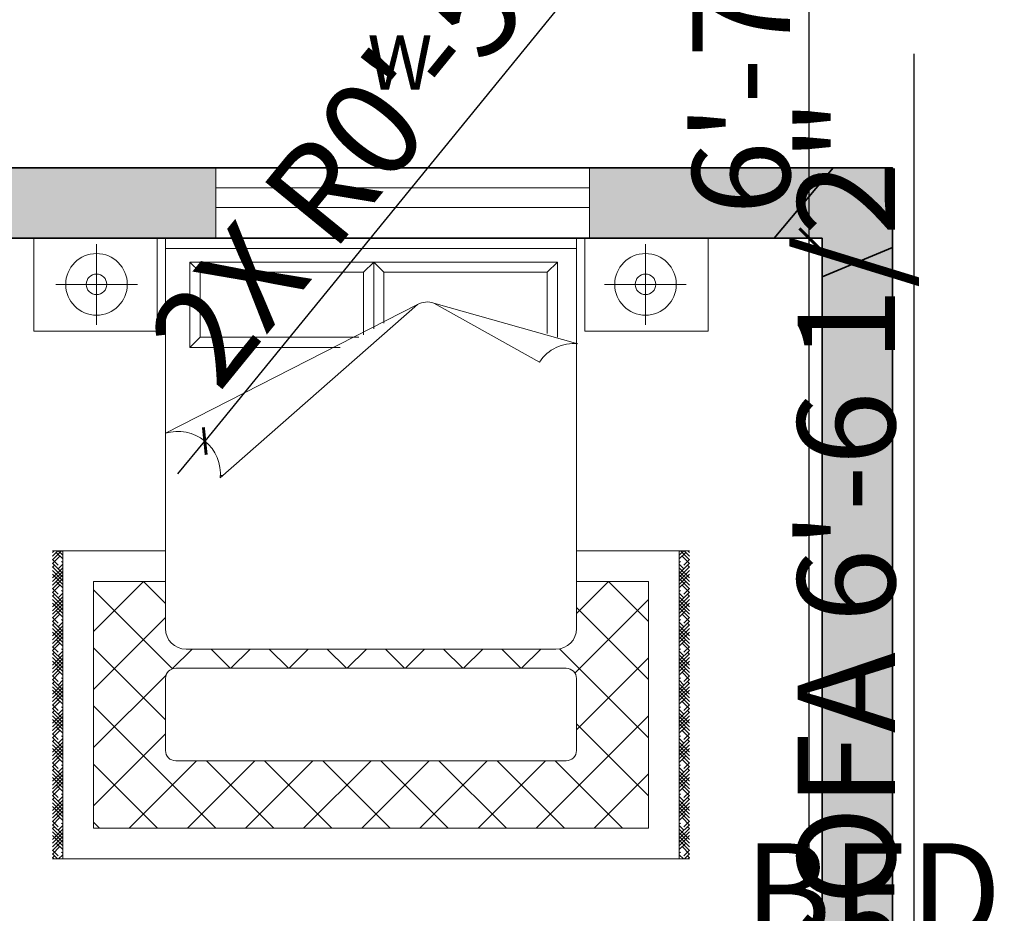
# Model space of a CAD drawing. Units: inches. Extents: x 1858 to 2399, y 1317 to 1943.
# Tile 6 of 8: x 2162 to 2288, y 1742 to 1856. Entities that reach past the tile are written whole.
import ezdxf

# ---------------------------------------------------------------- set-up
doc = ezdxf.new("R2010")
doc.units = ezdxf.units.IN
for name, color, linetype, lineweight in [('A-ANNO-DIMS', 2, 'Continuous', 18), ('A-ANNO-TEXT', 7, 'Continuous', 18), ('A-COLS', 7, 'Continuous', 35), ('A-COLS-PATT', 5, 'Continuous', 13), ('A-WALL', 7, 'Continuous', 35), ('A-WALL-PATT', 1, 'Continuous', 13), ('beds', 15, 'Continuous', 18), ('window', 4, 'Continuous', 18)]:
    doc.layers.add(name, color=color, linetype=linetype, lineweight=lineweight)
doc.styles.get("Standard").update_dxf_attribs({"font": 'arial.ttf'})
doc.dimstyles.new('ISO-25', dxfattribs={"dimtxt": 12.5, "dimasz": 2.5, "dimexe": 1.25, "dimexo": 0.625, "dimtad": 1, "dimdec": 0, "dimlunit": 4, "dimtxsty": 'Standard', "dimblk": 'ARCHTICK', "dimcen": 2.5, "dimse1": 1, "dimse2": 1, "dimclrd": 3, "dimclrt": 4, "dimadec": 0, "dimazin": 0, "dimtfac": 1, "dimtdec": 0, "dimtmove": 0, "dimatfit": 3, "dimfxl": 1, "dimarcsym": 0})

# ---------------------------------------------------------------- blocks, each defined once
blk = doc.blocks.new('A$C4CB008C5')
for p, q in [((0, 3.0188), (0.6, 3.0188)), ((0, 2.5688), (0, 3.0188)), ((0.6, 3.0188), (0.6, 2.5688)), ((0.6397, 1.1213), (0.6397, 3.0213)), ((0.6397, 3.0213), (2.6397, 3.0213)), ((2.6397, 3.0213), (2.6397, 1.1213)), ((3.2794, 3.0188), (2.6794, 3.0188)), ((2.6794, 3.0188), (2.6794, 2.5688)), ((3.2794, 2.5688), (3.2794, 3.0188)), ((0.3042, 2.5999), (0.3042, 2.9921)), ((0.6397, 2.9713), (2.6397, 2.9713)), ((2.9753, 2.5999), (2.9753, 2.9921)), ((0.7588, 2.9048), (2.5468, 2.9048)), ((0.7588, 2.4886), (0.7588, 2.9048)), ((0.7588, 2.9048), (0.8088, 2.8548)), ((1.6028, 2.8548), (1.6528, 2.9048)), ((1.6528, 2.9048), (1.6528, 2.5791)), ((1.6528, 2.9048), (1.7028, 2.8548)), ((2.4968, 2.8548), (2.5468, 2.9048)), ((2.5468, 2.9048), (2.5468, 2.5398)), ((0.8088, 2.8548), (1.6028, 2.8548)), ((0.8088, 2.5386), (0.8088, 2.8548)), ((1.6028, 2.8548), (1.6028, 2.5513)), ((1.7028, 2.8548), (1.7028, 2.6069)), ((1.7028, 2.8548), (2.4968, 2.8548)), ((2.4968, 2.8548), (2.4968, 2.5563)), ((0.1057, 2.796), (0.5033, 2.796)), ((3.1738, 2.796), (2.7761, 2.796)), ((0.6397, 2.0713), (1.866, 2.6977)), ((0.9063, 1.8539), (1.866, 2.6977)), ((1.946, 2.7052), (2.6461, 2.507)), ((1.946, 2.7052), (2.4598, 2.4178)), ((0.6, 2.5688), (0, 2.5688)), ((2.6794, 2.5688), (3.2794, 2.5688)), ((0.8088, 2.5386), (0.7588, 2.4886)), ((1.58, 2.5386), (0.8088, 2.5386)), ((1.4901, 2.4886), (0.7588, 2.4886)), ((0.9071, 1.8666), (0.9192, 1.8666)), ((0.0897, 1.5), (0.6397, 1.5)), ((0.0897, 1.491), (0.0987, 1.5)), ((0.0897, 1.4733), (0.1164, 1.5)), ((0.0897, 1.4557), (0.1341, 1.5)), ((0.1397, 1.4602), (0.1081, 1.4917)), ((0.1397, 1.4778), (0.1175, 1.5)), ((0.1397, 1.4955), (0.1352, 1.5)), ((0.1397, 0), (0.1397, 1.5)), ((2.6397, 1.5), (3.1897, 1.5)), ((3.1397, 1.4955), (3.1442, 1.5)), ((3.1397, 1.4778), (3.1619, 1.5)), ((3.1397, 1.5), (3.1397, 0)), ((3.1397, 1.4602), (3.1713, 1.4917)), ((3.1897, 1.4557), (3.1454, 1.5)), ((3.1897, 1.4733), (3.163, 1.5)), ((3.1897, 1.491), (3.1807, 1.5)), ((0.0904, 1.4741), (0.0897, 1.4748)), ((0.0897, 1.438), (0.1258, 1.4741)), ((0.117, 1.4299), (0.0897, 1.4571)), ((0.1397, 1.3894), (0.0897, 1.4394)), ((0.1397, 1.4425), (0.1346, 1.4475)), ((3.1397, 1.4425), (3.1448, 1.4475)), ((3.1397, 1.3894), (3.1897, 1.4394)), ((3.1897, 1.438), (3.1536, 1.4741)), ((3.1625, 1.4299), (3.1897, 1.4571)), ((3.189, 1.4741), (3.1897, 1.4748)), ((0.0897, 1.4203), (0.0993, 1.4299)), ((0.1397, 1.3718), (0.0897, 1.4218)), ((0.1397, 1.3541), (0.0897, 1.4041)), ((0.0897, 1.3496), (0.1397, 1.3996)), ((0.0904, 1.368), (0.1397, 1.4173)), ((0.117, 1.4122), (0.1397, 1.4349)), ((3.1625, 1.4122), (3.1397, 1.4349)), ((3.1397, 1.3718), (3.1897, 1.4218)), ((3.189, 1.368), (3.1397, 1.4173)), ((3.1397, 1.3541), (3.1897, 1.4041)), ((3.1897, 1.3496), (3.1397, 1.3996)), ((3.1897, 1.4203), (3.1801, 1.4299)), ((0.1397, 1.3364), (0.0897, 1.3864)), ((0.0897, 1.3319), (0.1397, 1.3819)), ((0.0897, 1.3142), (0.1397, 1.3642)), ((0.1397, 1.3187), (0.1081, 1.3503)), ((0.2897, 1.1076), (0.5321, 1.35)), ((0.2897, 0.15), (0.2897, 1.35)), ((0.2897, 1.35), (0.6397, 1.35)), ((0.6397, 1.243), (0.5327, 1.35)), ((2.6397, 1.1949), (2.7948, 1.35)), ((2.6397, 1.35), (2.9897, 1.35)), ((2.9897, 1.1557), (2.7955, 1.35)), ((2.9897, 1.35), (2.9897, 0.15)), ((3.1397, 1.3364), (3.1897, 1.3864)), ((3.1897, 1.3319), (3.1397, 1.3819)), ((3.1897, 1.3142), (3.1397, 1.3642)), ((3.1397, 1.3187), (3.1713, 1.3503)), ((0.0904, 1.3326), (0.0897, 1.3334)), ((0.0897, 1.2966), (0.1258, 1.3326)), ((0.117, 1.2885), (0.0897, 1.3157)), ((0.1397, 1.248), (0.0897, 1.298)), ((0.117, 1.2708), (0.1397, 1.2935)), ((0.1397, 1.3011), (0.1346, 1.3061)), ((0.6743, 0.9255), (0.2897, 1.3102)), ((3.1397, 1.3011), (3.1448, 1.3061)), ((3.1397, 1.248), (3.1897, 1.298)), ((3.1625, 1.2708), (3.1397, 1.2935)), ((3.1897, 1.2966), (3.1536, 1.3326)), ((3.1625, 1.2885), (3.1897, 1.3157)), ((3.189, 1.3326), (3.1897, 1.3334)), ((0.0897, 1.2789), (0.0993, 1.2885)), ((0.1397, 1.2303), (0.0897, 1.2803)), ((0.1397, 1.2127), (0.0897, 1.2627)), ((0.0897, 1.2082), (0.1397, 1.2582)), ((0.0904, 1.2266), (0.1397, 1.2758)), ((2.6321, 0.9045), (2.9897, 1.2621)), ((3.1397, 1.2303), (3.1897, 1.2803)), ((3.189, 1.2266), (3.1397, 1.2758)), ((3.1397, 1.2127), (3.1897, 1.2627)), ((3.1897, 1.2082), (3.1397, 1.2582)), ((3.1897, 1.2789), (3.1801, 1.2885)), ((0.1397, 1.195), (0.0897, 1.245)), ((0.0897, 1.1905), (0.1397, 1.2405)), ((0.0897, 1.1728), (0.1397, 1.2228)), ((0.1397, 1.1773), (0.1081, 1.2089)), ((2.9897, 0.8729), (2.6397, 1.2229)), ((3.1397, 1.195), (3.1897, 1.245)), ((3.1897, 1.1905), (3.1397, 1.2405)), ((3.1897, 1.1728), (3.1397, 1.2228)), ((3.1397, 1.1773), (3.1713, 1.2089)), ((0.0904, 1.1912), (0.0897, 1.192)), ((0.0897, 1.1551), (0.1258, 1.1912)), ((0.117, 1.147), (0.0897, 1.1743)), ((0.1397, 1.1066), (0.0897, 1.1566)), ((0.117, 1.1294), (0.1397, 1.1521)), ((0.1397, 1.1596), (0.1346, 1.1647)), ((0.2897, 0.8248), (0.6397, 1.1748)), ((3.1397, 1.1596), (3.1448, 1.1647)), ((3.1397, 1.1066), (3.1897, 1.1566)), ((3.1625, 1.1294), (3.1397, 1.1521)), ((3.1897, 1.1551), (3.1536, 1.1912)), ((3.1625, 1.147), (3.1897, 1.1743)), ((3.189, 1.1912), (3.1897, 1.192)), ((0.0897, 1.1375), (0.0993, 1.147)), ((0.1397, 1.0889), (0.0897, 1.1389)), ((0.1397, 1.0712), (0.0897, 1.1212)), ((0.0897, 1.0667), (0.1397, 1.1167)), ((0.1397, 1.0536), (0.0897, 1.1036)), ((0.0904, 1.0852), (0.1397, 1.1344)), ((3.1397, 1.0889), (3.1897, 1.1389)), ((3.189, 1.0852), (3.1397, 1.1344)), ((3.1397, 1.0712), (3.1897, 1.1212)), ((3.1897, 1.0667), (3.1397, 1.1167)), ((3.1397, 1.0536), (3.1897, 1.1036)), ((3.1897, 1.1375), (3.1801, 1.147)), ((0.0897, 1.0491), (0.1397, 1.0991)), ((0.0897, 1.0314), (0.1397, 1.0814)), ((0.1397, 1.0359), (0.1081, 1.0675)), ((3.1897, 1.0491), (3.1397, 1.0991)), ((3.1897, 1.0314), (3.1397, 1.0814)), ((3.1397, 1.0359), (3.1713, 1.0675)), ((0.0904, 1.0498), (0.0897, 1.0505)), ((0.0897, 1.0137), (0.1258, 1.0498)), ((0.117, 1.0056), (0.0897, 1.0329)), ((0.1397, 0.9652), (0.0897, 1.0152)), ((0.117, 0.9879), (0.1397, 1.0107)), ((0.1397, 1.0182), (0.1346, 1.0233)), ((0.6397, 0.6773), (0.2897, 1.0273)), ((0.6727, 0.925), (0.769, 1.0213)), ((2.5397, 1.0213), (0.7397, 1.0213)), ((0.9548, 0.9279), (0.8614, 1.0213)), ((0.9585, 0.9279), (1.0519, 1.0213)), ((1.2376, 0.9279), (1.1443, 1.0213)), ((1.2414, 0.9279), (1.3347, 1.0213)), ((1.5205, 0.9279), (1.4271, 1.0213)), ((1.5242, 0.9279), (1.6176, 1.0213)), ((1.8033, 0.9279), (1.71, 1.0213)), ((1.8071, 0.9279), (1.9004, 1.0213)), ((2.0861, 0.9279), (1.9928, 1.0213)), ((2.0899, 0.9279), (2.1832, 1.0213)), ((2.369, 0.9279), (2.2757, 1.0213)), ((2.3727, 0.9279), (2.4661, 1.0213)), ((2.9897, 0.5901), (2.557, 1.0228)), ((3.1397, 1.0182), (3.1448, 1.0233)), ((3.1397, 0.9652), (3.1897, 1.0152)), ((3.1625, 0.9879), (3.1397, 1.0107)), ((3.1897, 1.0137), (3.1536, 1.0498)), ((3.1625, 1.0056), (3.1897, 1.0329)), ((3.189, 1.0498), (3.1897, 1.0505)), ((0.0897, 0.996), (0.0993, 1.0056)), ((0.1397, 0.9475), (0.0897, 0.9975)), ((0.1397, 0.9298), (0.0897, 0.9798)), ((0.0897, 0.9253), (0.1397, 0.9753)), ((0.1397, 0.9121), (0.0897, 0.9621)), ((0.0904, 0.9437), (0.1397, 0.993)), ((2.6397, 0.6292), (2.9897, 0.9792)), ((3.1397, 0.9475), (3.1897, 0.9975)), ((3.189, 0.9437), (3.1397, 0.993)), ((3.1397, 0.9298), (3.1897, 0.9798)), ((3.1897, 0.9253), (3.1397, 0.9753)), ((3.1397, 0.9121), (3.1897, 0.9621)), ((3.1897, 0.996), (3.1801, 1.0056)), ((0.0897, 0.9076), (0.1397, 0.9576)), ((0.0897, 0.89), (0.1397, 0.94)), ((0.1397, 0.8945), (0.1081, 0.9261)), ((0.6897, 0.9279), (2.5897, 0.9279)), ((3.1897, 0.9076), (3.1397, 0.9576)), ((3.1897, 0.89), (3.1397, 0.94)), ((3.1397, 0.8945), (3.1713, 0.9261)), ((0.0904, 0.9084), (0.0897, 0.9091)), ((0.0897, 0.8723), (0.1258, 0.9084)), ((0.117, 0.8642), (0.0897, 0.8914)), ((0.1397, 0.8238), (0.0897, 0.8738)), ((0.0897, 0.8546), (0.0993, 0.8642)), ((0.117, 0.8465), (0.1397, 0.8693)), ((0.1397, 0.8768), (0.1346, 0.8819)), ((0.2897, 0.542), (0.6427, 0.8949)), ((0.6397, 0.8779), (0.6397, 0.5279)), ((2.6397, 0.8779), (2.6397, 0.5279)), ((3.1397, 0.8768), (3.1448, 0.8819)), ((3.1397, 0.8238), (3.1897, 0.8738)), ((3.1625, 0.8465), (3.1397, 0.8693)), ((3.1897, 0.8723), (3.1536, 0.9084)), ((3.1625, 0.8642), (3.1897, 0.8914)), ((3.1897, 0.8546), (3.1801, 0.8642)), ((3.189, 0.9084), (3.1897, 0.9091)), ((0.1397, 0.8061), (0.0897, 0.8561)), ((0.1397, 0.7884), (0.0897, 0.8384)), ((0.0897, 0.7839), (0.1397, 0.8339)), ((0.1397, 0.7707), (0.0897, 0.8207)), ((0.0897, 0.7662), (0.1397, 0.8162)), ((0.0904, 0.8023), (0.1397, 0.8516)), ((3.1397, 0.8061), (3.1897, 0.8561)), ((3.189, 0.8023), (3.1397, 0.8516)), ((3.1397, 0.7884), (3.1897, 0.8384)), ((3.1897, 0.7839), (3.1397, 0.8339)), ((3.1397, 0.7707), (3.1897, 0.8207)), ((3.1897, 0.7662), (3.1397, 0.8162)), ((0.0897, 0.7485), (0.1397, 0.7985)), ((0.0904, 0.767), (0.0897, 0.7677)), ((0.0897, 0.7309), (0.1258, 0.767)), ((0.1397, 0.7531), (0.1081, 0.7846)), ((3.1897, 0.7485), (3.1397, 0.7985)), ((3.1397, 0.7531), (3.1713, 0.7846)), ((3.1897, 0.7309), (3.1536, 0.767)), ((3.189, 0.767), (3.1897, 0.7677)), ((0.117, 0.7228), (0.0897, 0.75)), ((0.1397, 0.6823), (0.0897, 0.7323)), ((0.0897, 0.7132), (0.0993, 0.7228)), ((0.117, 0.7051), (0.1397, 0.7278)), ((0.1397, 0.7354), (0.1346, 0.7404)), ((0.8842, 0.15), (0.2897, 0.7445)), ((3.1397, 0.7354), (3.1448, 0.7404)), ((3.1397, 0.6823), (3.1897, 0.7323)), ((3.1625, 0.7051), (3.1397, 0.7278)), ((3.1625, 0.7228), (3.1897, 0.75)), ((3.1897, 0.7132), (3.1801, 0.7228)), ((0.1397, 0.6647), (0.0897, 0.7147)), ((0.1397, 0.647), (0.0897, 0.697)), ((0.0897, 0.6425), (0.1397, 0.6925)), ((0.1397, 0.6293), (0.0897, 0.6793)), ((0.0897, 0.6248), (0.1397, 0.6748)), ((0.0904, 0.6609), (0.1397, 0.7102)), ((2.4433, 0.15), (2.9897, 0.6964)), ((3.1397, 0.6647), (3.1897, 0.7147)), ((3.189, 0.6609), (3.1397, 0.7102)), ((3.1397, 0.647), (3.1897, 0.697)), ((3.1897, 0.6425), (3.1397, 0.6925)), ((3.1397, 0.6293), (3.1897, 0.6793)), ((3.1897, 0.6248), (3.1397, 0.6748)), ((0.0897, 0.6071), (0.1397, 0.6571)), ((0.0904, 0.6255), (0.0897, 0.6263)), ((0.0897, 0.5894), (0.1258, 0.6255)), ((0.1397, 0.6116), (0.1081, 0.6432)), ((2.9897, 0.3072), (2.6397, 0.6572)), ((3.1897, 0.6071), (3.1397, 0.6571)), ((3.1397, 0.6116), (3.1713, 0.6432)), ((3.1897, 0.5894), (3.1536, 0.6255)), ((3.189, 0.6255), (3.1897, 0.6263)), ((0.117, 0.5813), (0.0897, 0.6086)), ((0.1397, 0.5409), (0.0897, 0.5909)), ((0.0897, 0.5718), (0.0993, 0.5813)), ((0.117, 0.5637), (0.1397, 0.5864)), ((0.1397, 0.594), (0.1346, 0.599)), ((0.2897, 0.2591), (0.6397, 0.6091)), ((3.1397, 0.594), (3.1448, 0.599)), ((3.1397, 0.5409), (3.1897, 0.5909)), ((3.1625, 0.5637), (3.1397, 0.5864)), ((3.1625, 0.5813), (3.1897, 0.6086)), ((3.1897, 0.5718), (3.1801, 0.5813)), ((0.1397, 0.5232), (0.0897, 0.5732)), ((0.1397, 0.5056), (0.0897, 0.5556)), ((0.0897, 0.5011), (0.1397, 0.5511)), ((0.1397, 0.4879), (0.0897, 0.5379)), ((0.0897, 0.4834), (0.1397, 0.5334)), ((0.0904, 0.5195), (0.1397, 0.5687)), ((3.1397, 0.5232), (3.1897, 0.5732)), ((3.189, 0.5195), (3.1397, 0.5687)), ((3.1397, 0.5056), (3.1897, 0.5556)), ((3.1897, 0.5011), (3.1397, 0.5511)), ((3.1397, 0.4879), (3.1897, 0.5379)), ((3.1897, 0.4834), (3.1397, 0.5334)), ((0.0897, 0.4657), (0.1397, 0.5157)), ((0.0904, 0.4841), (0.0897, 0.4849)), ((0.0897, 0.448), (0.1258, 0.4841)), ((0.1397, 0.4702), (0.1081, 0.5018)), ((3.1897, 0.4657), (3.1397, 0.5157)), ((3.1397, 0.4702), (3.1713, 0.5018)), ((3.1897, 0.448), (3.1536, 0.4841)), ((3.189, 0.4841), (3.1897, 0.4849)), ((0.117, 0.4399), (0.0897, 0.4672)), ((0.1397, 0.3995), (0.0897, 0.4495)), ((0.0897, 0.4303), (0.0993, 0.4399)), ((0.1397, 0.3818), (0.0897, 0.4318)), ((0.117, 0.4222), (0.1397, 0.445)), ((0.1397, 0.4525), (0.1346, 0.4576)), ((0.6013, 0.15), (0.2897, 0.4616)), ((0.4634, 0.15), (0.7914, 0.4779)), ((0.6897, 0.4779), (2.5897, 0.4779)), ((0.7463, 0.15), (1.0742, 0.4779)), ((1.167, 0.15), (0.8391, 0.4779)), ((1.0291, 0.15), (1.3571, 0.4779)), ((1.4499, 0.15), (1.1219, 0.4779)), ((1.312, 0.15), (1.6399, 0.4779)), ((1.7327, 0.15), (1.4048, 0.4779)), ((1.5948, 0.15), (1.9227, 0.4779)), ((2.0156, 0.15), (1.6876, 0.4779)), ((1.8777, 0.15), (2.2056, 0.4779)), ((2.2984, 0.15), (1.9705, 0.4779)), ((2.1605, 0.15), (2.4884, 0.4779)), ((2.5812, 0.15), (2.2533, 0.4779)), ((2.8641, 0.15), (2.5361, 0.4779)), ((3.1397, 0.4525), (3.1448, 0.4576)), ((3.1397, 0.3995), (3.1897, 0.4495)), ((3.1625, 0.4222), (3.1397, 0.445)), ((3.1397, 0.3818), (3.1897, 0.4318)), ((3.1625, 0.4399), (3.1897, 0.4672)), ((3.1897, 0.4303), (3.1801, 0.4399)), ((0.1397, 0.3641), (0.0897, 0.4141)), ((0.0897, 0.3596), (0.1397, 0.4096)), ((0.1397, 0.3465), (0.0897, 0.3965)), ((0.0897, 0.342), (0.1397, 0.392)), ((0.0904, 0.3781), (0.1397, 0.4273)), ((2.7262, 0.15), (2.9897, 0.4135)), ((3.189, 0.3781), (3.1397, 0.4273)), ((3.1397, 0.3641), (3.1897, 0.4141)), ((3.1897, 0.3596), (3.1397, 0.4096)), ((3.1397, 0.3465), (3.1897, 0.3965)), ((3.1897, 0.342), (3.1397, 0.392)), ((0.0897, 0.3243), (0.1397, 0.3743)), ((0.0904, 0.3427), (0.0897, 0.3434)), ((0.0897, 0.3066), (0.1258, 0.3427)), ((0.1397, 0.3288), (0.1081, 0.3604)), ((3.1897, 0.3243), (3.1397, 0.3743)), ((3.1397, 0.3288), (3.1713, 0.3604)), ((3.1897, 0.3066), (3.1536, 0.3427)), ((3.189, 0.3427), (3.1897, 0.3434)), ((0.117, 0.2985), (0.0897, 0.3258)), ((0.1397, 0.2581), (0.0897, 0.3081)), ((0.0897, 0.2889), (0.0993, 0.2985)), ((0.1397, 0.2404), (0.0897, 0.2904)), ((0.117, 0.2808), (0.1397, 0.3036)), ((0.1397, 0.3111), (0.1346, 0.3162)), ((3.1397, 0.3111), (3.1448, 0.3162)), ((3.1397, 0.2581), (3.1897, 0.3081)), ((3.1625, 0.2808), (3.1397, 0.3036)), ((3.1397, 0.2404), (3.1897, 0.2904)), ((3.1625, 0.2985), (3.1897, 0.3258)), ((3.1897, 0.2889), (3.1801, 0.2985)), ((0.1397, 0.2227), (0.0897, 0.2727)), ((0.0897, 0.2182), (0.1397, 0.2682)), ((0.1397, 0.205), (0.0897, 0.255)), ((0.0897, 0.2005), (0.1397, 0.2505)), ((0.0904, 0.2366), (0.1397, 0.2859)), ((3.189, 0.2366), (3.1397, 0.2859)), ((3.1397, 0.2227), (3.1897, 0.2727)), ((3.1897, 0.2182), (3.1397, 0.2682)), ((3.1397, 0.205), (3.1897, 0.255)), ((3.1897, 0.2005), (3.1397, 0.2505)), ((0.0897, 0.1829), (0.1397, 0.2329)), ((0.0904, 0.2013), (0.0897, 0.202)), ((0.0897, 0.1652), (0.1258, 0.2013)), ((0.1397, 0.1874), (0.1081, 0.219)), ((3.1897, 0.1829), (3.1397, 0.2329)), ((3.1397, 0.1874), (3.1713, 0.219)), ((3.1897, 0.1652), (3.1536, 0.2013)), ((3.189, 0.2013), (3.1897, 0.202)), ((0.117, 0.1571), (0.0897, 0.1843)), ((0.1397, 0.1167), (0.0897, 0.1667)), ((0.0897, 0.1475), (0.0993, 0.1571)), ((0.1397, 0.099), (0.0897, 0.149)), ((0.0904, 0.0952), (0.1397, 0.1445)), ((0.117, 0.1394), (0.1397, 0.1621)), ((0.1397, 0.1697), (0.1346, 0.1748)), ((0.3185, 0.15), (0.2897, 0.1788)), ((2.9897, 0.15), (0.2897, 0.15)), ((3.1397, 0.1697), (3.1448, 0.1748)), ((3.1397, 0.1167), (3.1897, 0.1667)), ((3.1625, 0.1394), (3.1397, 0.1621)), ((3.1397, 0.099), (3.1897, 0.149)), ((3.189, 0.0952), (3.1397, 0.1445)), ((3.1625, 0.1571), (3.1897, 0.1843)), ((3.1897, 0.1475), (3.1801, 0.1571)), ((0.1397, 0.0813), (0.0897, 0.1313)), ((0.0897, 0.0768), (0.1397, 0.1268)), ((0.1397, 0.0636), (0.0897, 0.1136)), ((0.0897, 0.0591), (0.1397, 0.1091)), ((3.1397, 0.0813), (3.1897, 0.1313)), ((3.1897, 0.0768), (3.1397, 0.1268)), ((3.1397, 0.0636), (3.1897, 0.1136)), ((3.1897, 0.0591), (3.1397, 0.1091)), ((0.0897, 0.0414), (0.1397, 0.0914)), ((0.0904, 0.0599), (0.0897, 0.0606)), ((0.0897, 0.0238), (0.1258, 0.0599)), ((0.1397, 0.0459), (0.1081, 0.0775)), ((3.1897, 0.0414), (3.1397, 0.0914)), ((3.1397, 0.0459), (3.1713, 0.0775)), ((3.1897, 0.0238), (3.1536, 0.0599)), ((3.189, 0.0599), (3.1897, 0.0606)), ((0.117, 0.0157), (0.0897, 0.0429)), ((0.1149, 0), (0.0897, 0.0252)), ((0.0897, 0.0061), (0.0993, 0.0157)), ((0.0973, 0), (0.0897, 0.0076)), ((0.119, 0), (0.1397, 0.0207)), ((0.1397, 0.0283), (0.1346, 0.0333)), ((0.1367, 0), (0.1397, 0.0031)), ((3.1397, 0.0283), (3.1448, 0.0333)), ((3.1604, 0), (3.1397, 0.0207)), ((3.1428, 0), (3.1397, 0.0031)), ((3.1625, 0.0157), (3.1897, 0.0429)), ((3.1645, 0), (3.1897, 0.0252)), ((3.1897, 0.0061), (3.1801, 0.0157)), ((3.1822, 0), (3.1897, 0.0076)), ((0.0897, 0), (3.1897, 0))]:
    blk.add_line(p, q)
for centre, radius in [((0.3042, 2.796), 0.15), ((2.9753, 2.796), 0.15), ((0.3042, 2.796), 0.05), ((2.9753, 2.796), 0.05)]:
    blk.add_circle(centre, radius)
for centre, radius, start, end in [((1.9146, 2.6103), 0.1, 71.7215, 119.0799), ((2.626, 2.3098), 0.1982, 84.1725, 146.9889), ((0.7002, 1.8733), 0.207, 354.6422, 106.9775), ((0.7397, 1.1213), 0.1, 180, 270), ((2.5397, 1.1213), 0.1, 270, 0), ((0.6897, 0.8779), 0.05, 90, 180), ((2.5897, 0.8779), 0.05, 0, 90), ((0.6897, 0.5279), 0.05, 180, 270), ((2.5897, 0.5279), 0.05, 270, 0)]:
    blk.add_arc(centre, radius, start, end)
blk = doc.blocks.new('_ArchTick')
at = {"color": 0, "linetype": 'ByBlock', "const_width": 0.15}
blk.add_lwpolyline([(-0.5, -0.5), (0.5, 0.5)], dxfattribs=at)
blk = doc.blocks.new('*D13')
at = {"layer": 'A-ANNO-DIMS', "color": 0, "lineweight": -2, "transparency": 16777216}
blk.add_line((2316.13, 1837.34), (2316.13, 1357.34), dxfattribs=at)
at = {"layer": 'Defpoints', "color": 0, "transparency": 16777216}
for p in [(2273.38, 1837.34), (2273.38, 1357.34), (2316.13, 1357.34)]:
    blk.add_point(p, dxfattribs=at)
at = {"layer": 'A-ANNO-DIMS', "color": 0, "lineweight": -2, "transparency": 16777216, "xscale": 2.5, "yscale": 2.5, "zscale": 2.5}
for p, rotation in [((2316.13, 1837.34), 90), ((2316.13, 1357.34), 270)]:
    blk.add_blockref('_ArchTick', p, dxfattribs=dict(at, rotation=rotation))
at = {"layer": 'A-ANNO-DIMS', "color": 0, "transparency": 16777216, "insert": (2309.12, 1597.34), "char_height": 12.5, "attachment_point": 5, "rotation": 90}
blk.add_mtext("40'", dxfattribs=at)
blk = doc.blocks.new('*D14')
at = {"layer": 'A-ANNO-DIMS', "color": 0, "lineweight": -2, "transparency": 16777216}
blk.add_line((1913.38, 1886.42), (2273.38, 1886.42), dxfattribs=at)
at = {"layer": 'Defpoints', "color": 0, "transparency": 16777216}
for p in [(2273.38, 1886.42), (1913.38, 1826.41), (2273.38, 1827.14)]:
    blk.add_point(p, dxfattribs=at)
at = {"layer": 'A-ANNO-DIMS', "color": 0, "lineweight": -2, "transparency": 16777216, "xscale": 2.5, "yscale": 2.5, "zscale": 2.5, "rotation": 180}
blk.add_blockref('_ArchTick', (1913.38, 1886.42), dxfattribs=at)
at = {"layer": 'A-ANNO-DIMS', "color": 0, "lineweight": -2, "transparency": 16777216, "xscale": 2.5, "yscale": 2.5, "zscale": 2.5}
blk.add_blockref('_ArchTick', (2273.38, 1886.42), dxfattribs=at)
at = {"layer": 'A-ANNO-DIMS', "color": 0, "transparency": 16777216, "insert": (2093.38, 1893.43), "char_height": 12.5, "attachment_point": 5}
blk.add_mtext("30'", dxfattribs=at)
blk = doc.blocks.new('*D15')
at = {"layer": 'A-ANNO-DIMS', "color": 3, "lineweight": -2, "transparency": 16777216}
for p, q in [((2163.42, 1735.85), (2249.76, 1735.85)), ((2249.76, 1735.85), (2399.03, 1735.85))]:
    blk.add_line(p, q, dxfattribs=at)
at = {"layer": 'Defpoints', "color": 0, "transparency": 16777216}
for p in [(2163.42, 1748.8), (2249.76, 1748.8), (2249.76, 1735.85)]:
    blk.add_point(p, dxfattribs=at)
at = {"layer": 'A-ANNO-DIMS', "color": 3, "lineweight": -2, "transparency": 16777216, "xscale": 2.5, "yscale": 2.5, "zscale": 2.5, "rotation": 180}
blk.add_blockref('_ArchTick', (2163.42, 1735.85), dxfattribs=at)
at = {"layer": 'A-ANNO-DIMS', "color": 3, "lineweight": -2, "transparency": 16777216, "xscale": 2.5, "yscale": 2.5, "zscale": 2.5}
blk.add_blockref('_ArchTick', (2249.76, 1735.85), dxfattribs=at)
at = {"layer": 'A-ANNO-DIMS', "color": 4, "transparency": 16777216, "insert": (2325.64, 1742.94), "char_height": 12.5, "attachment_point": 5}
blk.add_mtext('BED 7\'-2 1/2" TYP.', dxfattribs=at)
blk = doc.blocks.new('*D16')
at = {"layer": 'A-ANNO-DIMS', "color": 3, "lineweight": -2, "transparency": 16777216}
for p, q in [((2262.71, 1828.34), (2262.71, 1937.48)), ((2262.71, 1748.8), (2262.71, 1828.34))]:
    blk.add_line(p, q, dxfattribs=at)
at = {"layer": 'Defpoints', "color": 0, "transparency": 16777216}
for p in [(2249.76, 1828.34), (2262.71, 1828.34), (2249.76, 1748.8)]:
    blk.add_point(p, dxfattribs=at)
at = {"layer": 'A-ANNO-DIMS', "color": 3, "lineweight": -2, "transparency": 16777216, "xscale": 2.5, "yscale": 2.5, "zscale": 2.5}
for p, rotation in [((2262.71, 1828.34), 90), ((2262.71, 1748.8), 270)]:
    blk.add_blockref('_ArchTick', p, dxfattribs=dict(at, rotation=rotation))
at = {"layer": 'A-ANNO-DIMS', "color": 4, "transparency": 16777216, "insert": (2255.62, 1884.16), "char_height": 12.5, "attachment_point": 5, "rotation": 90}
blk.add_mtext('6\'-7 1/2" TYP.', dxfattribs=at)
blk = doc.blocks.new('*D17')
at = {"layer": 'A-ANNO-DIMS', "color": 3, "lineweight": -2, "transparency": 16777216}
for p, q in [((2276.18, 1653.07), (2276.18, 1851.95)), ((2276.18, 1574.39), (2276.18, 1653.07))]:
    blk.add_line(p, q, dxfattribs=at)
at = {"layer": 'Defpoints', "color": 0, "transparency": 16777216}
for p in [(2264.38, 1653.07), (2276.18, 1653.07), (2264.38, 1574.39)]:
    blk.add_point(p, dxfattribs=at)
at = {"layer": 'A-ANNO-DIMS', "color": 3, "lineweight": -2, "transparency": 16777216, "xscale": 2.5, "yscale": 2.5, "zscale": 2.5}
for p, rotation in [((2276.18, 1653.07), 90), ((2276.18, 1574.39), 270)]:
    blk.add_blockref('_ArchTick', p, dxfattribs=dict(at, rotation=rotation))
at = {"layer": 'A-ANNO-DIMS', "color": 4, "transparency": 16777216, "insert": (2269.09, 1753.76), "char_height": 12.5, "attachment_point": 5, "rotation": 90}
blk.add_mtext('CORNER SOFA 6\'-6 1/2"', dxfattribs=at)
blk = doc.blocks.new('*D35')
at = {"layer": 'A-ANNO-DIMS', "color": 3, "lineweight": -2, "transparency": 16777216}
for p, q in [((2107.67, 1917.54), (2131.33, 1917.54)), ((2131.33, 1917.54), (2205.97, 1917.54))]:
    blk.add_line(p, q, dxfattribs=at)
at = {"layer": 'Defpoints', "color": 0, "transparency": 16777216}
for p in [(2131.33, 1917.54), (2107.67, 1837.34), (2131.33, 1837.34)]:
    blk.add_point(p, dxfattribs=at)
at = {"layer": 'A-ANNO-DIMS', "color": 3, "lineweight": -2, "transparency": 16777216, "xscale": 2.5, "yscale": 2.5, "zscale": 2.5, "rotation": 180}
blk.add_blockref('_ArchTick', (2107.67, 1917.54), dxfattribs=at)
at = {"layer": 'A-ANNO-DIMS', "color": 3, "lineweight": -2, "transparency": 16777216, "xscale": 2.5, "yscale": 2.5, "zscale": 2.5}
blk.add_blockref('_ArchTick', (2131.33, 1917.54), dxfattribs=at)
at = {"layer": 'A-ANNO-DIMS', "color": 4, "transparency": 16777216, "insert": (2169.9, 1924.63), "char_height": 12.5, "attachment_point": 5}
blk.add_mtext('1\'-11 1/2"', dxfattribs=at)
blk = doc.blocks.new('*D36')
at = {"layer": 'A-ANNO-DIMS', "color": 3, "lineweight": -2, "transparency": 16777216}
for p, q in [((2131.33, 1917.54), (2186.7, 1917.54)), ((2186.7, 1917.54), (2253.31, 1917.54))]:
    blk.add_line(p, q, dxfattribs=at)
at = {"layer": 'Defpoints', "color": 0, "transparency": 16777216}
for p in [(2186.7, 1917.54), (2131.33, 1837.34), (2186.7, 1837.34)]:
    blk.add_point(p, dxfattribs=at)
at = {"layer": 'A-ANNO-DIMS', "color": 3, "lineweight": -2, "transparency": 16777216, "xscale": 2.5, "yscale": 2.5, "zscale": 2.5, "rotation": 180}
blk.add_blockref('_ArchTick', (2131.33, 1917.54), dxfattribs=at)
at = {"layer": 'A-ANNO-DIMS', "color": 3, "lineweight": -2, "transparency": 16777216, "xscale": 2.5, "yscale": 2.5, "zscale": 2.5}
blk.add_blockref('_ArchTick', (2186.7, 1917.54), dxfattribs=at)
at = {"layer": 'A-ANNO-DIMS', "color": 4, "transparency": 16777216, "insert": (2221.25, 1924.63), "char_height": 12.5, "attachment_point": 5}
blk.add_mtext('4\'-7 1/2"', dxfattribs=at)
blk = doc.blocks.new('*D37')
at = {"layer": 'A-ANNO-DIMS', "color": 3, "lineweight": -2, "transparency": 16777216}
blk.add_line((2186.7, 1917.54), (2234.56, 1917.54), dxfattribs=at)
at = {"layer": 'Defpoints', "color": 0, "transparency": 16777216}
for p in [(2234.56, 1917.54), (2186.7, 1837.34), (2234.56, 1837.34)]:
    blk.add_point(p, dxfattribs=at)
at = {"layer": 'A-ANNO-DIMS', "color": 3, "lineweight": -2, "transparency": 16777216, "xscale": 2.5, "yscale": 2.5, "zscale": 2.5, "rotation": 180}
blk.add_blockref('_ArchTick', (2186.7, 1917.54), dxfattribs=at)
at = {"layer": 'A-ANNO-DIMS', "color": 3, "lineweight": -2, "transparency": 16777216, "xscale": 2.5, "yscale": 2.5, "zscale": 2.5}
blk.add_blockref('_ArchTick', (2234.56, 1917.54), dxfattribs=at)
at = {"layer": 'A-ANNO-DIMS', "color": 4, "transparency": 16777216, "insert": (2210.63, 1924.55), "char_height": 12.5, "attachment_point": 5}
blk.add_mtext('4\'-0"', dxfattribs=at)
blk = doc.blocks.new('*D38')
at = {"layer": 'A-ANNO-DIMS', "color": 3, "lineweight": -2, "transparency": 16777216}
blk.add_line((2234.56, 1917.54), (2273.38, 1917.54), dxfattribs=at)
at = {"layer": 'Defpoints', "color": 0, "transparency": 16777216}
for p in [(2273.38, 1917.54), (2234.56, 1837.34), (2273.38, 1837.34)]:
    blk.add_point(p, dxfattribs=at)
at = {"layer": 'A-ANNO-DIMS', "color": 3, "lineweight": -2, "transparency": 16777216, "xscale": 2.5, "yscale": 2.5, "zscale": 2.5, "rotation": 180}
blk.add_blockref('_ArchTick', (2234.56, 1917.54), dxfattribs=at)
at = {"layer": 'A-ANNO-DIMS', "color": 3, "lineweight": -2, "transparency": 16777216, "xscale": 2.5, "yscale": 2.5, "zscale": 2.5}
blk.add_blockref('_ArchTick', (2273.38, 1917.54), dxfattribs=at)
at = {"layer": 'A-ANNO-DIMS', "color": 4, "transparency": 16777216, "insert": (2253.97, 1924.55), "char_height": 12.5, "attachment_point": 5}
blk.add_mtext('3\'-3"', dxfattribs=at)
blk = doc.blocks.new('*D50')
at = {"layer": 'A-ANNO-DIMS', "color": 3, "lineweight": -2, "transparency": 16777216}
for p, q in [((2097.46, 1917.54), (2127.41, 1917.54)), ((2127.41, 1917.54), (2164.6, 1917.54))]:
    blk.add_line(p, q, dxfattribs=at)
at = {"layer": 'Defpoints', "color": 0, "transparency": 16777216}
for p in [(2127.41, 1917.54), (2097.46, 1563.34), (2127.41, 1563.34)]:
    blk.add_point(p, dxfattribs=at)
at = {"layer": 'A-ANNO-DIMS', "color": 3, "lineweight": -2, "transparency": 16777216, "xscale": 2.5, "yscale": 2.5, "zscale": 2.5, "rotation": 180}
blk.add_blockref('_ArchTick', (2097.46, 1917.54), dxfattribs=at)
at = {"layer": 'A-ANNO-DIMS', "color": 3, "lineweight": -2, "transparency": 16777216, "xscale": 2.5, "yscale": 2.5, "zscale": 2.5}
blk.add_blockref('_ArchTick', (2127.41, 1917.54), dxfattribs=at)
at = {"layer": 'A-ANNO-DIMS', "color": 4, "transparency": 16777216, "insert": (2147.25, 1924.55), "char_height": 12.5, "attachment_point": 5}
blk.add_mtext('2\'-6"', dxfattribs=at)
blk = doc.blocks.new('*D51')
at = {"layer": 'A-ANNO-DIMS', "color": 3, "lineweight": -2, "transparency": 16777216}
for p, q in [((2127.41, 1917.54), (2171.86, 1917.54)), ((2171.86, 1917.54), (2237.95, 1917.54))]:
    blk.add_line(p, q, dxfattribs=at)
at = {"layer": 'Defpoints', "color": 0, "transparency": 16777216}
for p in [(2171.86, 1917.54), (2127.41, 1563.34), (2171.86, 1563.34)]:
    blk.add_point(p, dxfattribs=at)
at = {"layer": 'A-ANNO-DIMS', "color": 3, "lineweight": -2, "transparency": 16777216, "xscale": 2.5, "yscale": 2.5, "zscale": 2.5, "rotation": 180}
blk.add_blockref('_ArchTick', (2127.41, 1917.54), dxfattribs=at)
at = {"layer": 'A-ANNO-DIMS', "color": 3, "lineweight": -2, "transparency": 16777216, "xscale": 2.5, "yscale": 2.5, "zscale": 2.5}
blk.add_blockref('_ArchTick', (2171.86, 1917.54), dxfattribs=at)
at = {"layer": 'A-ANNO-DIMS', "color": 4, "transparency": 16777216, "insert": (2206.15, 1924.63), "char_height": 12.5, "attachment_point": 5}
blk.add_mtext('3\'-8 1/2"', dxfattribs=at)
blk = doc.blocks.new('*D52')
at = {"layer": 'A-ANNO-DIMS', "color": 3, "lineweight": -2, "transparency": 16777216}
blk.add_line((2171.86, 1917.54), (2220, 1917.54), dxfattribs=at)
at = {"layer": 'Defpoints', "color": 0, "transparency": 16777216}
for p in [(2220, 1917.54), (2171.86, 1563.34), (2220, 1563.34)]:
    blk.add_point(p, dxfattribs=at)
at = {"layer": 'A-ANNO-DIMS', "color": 3, "lineweight": -2, "transparency": 16777216, "xscale": 2.5, "yscale": 2.5, "zscale": 2.5, "rotation": 180}
blk.add_blockref('_ArchTick', (2171.86, 1917.54), dxfattribs=at)
at = {"layer": 'A-ANNO-DIMS', "color": 3, "lineweight": -2, "transparency": 16777216, "xscale": 2.5, "yscale": 2.5, "zscale": 2.5}
blk.add_blockref('_ArchTick', (2220, 1917.54), dxfattribs=at)
at = {"layer": 'A-ANNO-DIMS', "color": 4, "transparency": 16777216, "insert": (2195.93, 1924.55), "char_height": 12.5, "attachment_point": 5}
blk.add_mtext('4\'-0"', dxfattribs=at)
blk = doc.blocks.new('*D60')
at = {"layer": 'A-ANNO-DIMS', "color": 3, "lineweight": -2, "transparency": 16777216}
for p in [(2253.32, 1885.76), (2181.85, 1798.12)]:
    blk.add_line(p, (2185.3, 1802.34), dxfattribs=at)
at = {"layer": 'Defpoints', "color": 0, "transparency": 16777216}
for p in [(2185.3, 1802.34), (2181.85, 1798.12)]:
    blk.add_point(p, dxfattribs=at)
at = {"layer": 'A-ANNO-DIMS', "color": 3, "lineweight": -2, "transparency": 16777216, "xscale": 2.5, "yscale": 2.5, "zscale": 2.5, "rotation": 230.8077101952448}
blk.add_blockref('_ArchTick', (2185.3, 1802.34), dxfattribs=at)
at = {"layer": 'A-ANNO-DIMS', "color": 4, "transparency": 16777216, "insert": (2215.4, 1850.47), "char_height": 12.5, "attachment_point": 5, "rotation": 50.8077}
blk.add_mtext('2X R0\'-5 1/2"', dxfattribs=at)

msp = doc.modelspace()

# ---------------------------------------------------------------- hatches: boundary and pattern name
at = {"layer": 'A-COLS-PATT'}
h = msp.add_hatch(color=256, dxfattribs=at)
h.dxf.hatch_style = 1
h.paths.add_polyline_path([(1977.99, 1696.34), (1967.38, 1696.34), (1967.38, 1700.89), (1958.38, 1700.89), (1958.38, 1685.05), (1967.38, 1685.05), (1967.38, 1691.34), (1977.99, 1691.34)])
h.paths.add_polyline_path([(1967.38, 1571.83), (1958.38, 1571.83), (1958.38, 1559.34), (1967.38, 1559.34)])
h.paths.add_polyline_path([(1977.97, 1476.34), (1967.38, 1476.34), (1967.38, 1482.01), (1958.38, 1474.25), (1958.38, 1467.34), (1967.38, 1467.34)])
h.paths.add_polyline_path([(2096.38, 1473.96), (2087.38, 1481.51), (2087.38, 1476.34), (2084.48, 1476.34), (2089.85, 1467.34), (2096.38, 1467.34)])
h.paths.add_polyline_path([(2273.38, 1837.34), (2265.79, 1837.34), (2258.24, 1828.34), (2264.38, 1828.34), (2264.38, 1823.36), (2273.38, 1827.14)])
h.paths.add_polyline_path([(2097.64, 1837.34), (2082.58, 1837.34), (2082.58, 1828.34), (2097.64, 1828.34)])
h.paths.add_polyline_path([(1977.66, 1837.34), (1949.42, 1837.34), (1949.42, 1828.34), (1977.66, 1828.34)])
at = {"layer": 'A-WALL-PATT'}
h = msp.add_hatch(color=256, dxfattribs=at)
h.dxf.hatch_style = 1
h.paths.add_polyline_path([(1967.38, 1742.58), (1958.38, 1742.58), (1958.38, 1700.89), (1967.38, 1700.89)])
h.paths.add_polyline_path([(1967.38, 1685.05), (1958.38, 1685.05), (1958.38, 1672.42), (1967.38, 1672.42)], flags=17)
h.paths.add_polyline_path([(2092.38, 1643.34), (2087.38, 1643.34), (2063.38, 1643.34), (2063.38, 1691.34), (2087.38, 1691.34), (2092.38, 1691.34), (2092.38, 1696.34), (2087.38, 1696.34), (2005.38, 1696.34), (2005.38, 1691.34), (2058.38, 1691.34), (2058.38, 1643.34), (1967.38, 1643.34), (1967.38, 1652.51), (1958.38, 1652.51), (1958.38, 1625.4), (1967.38, 1625.4), (1967.38, 1638.34), (2087.38, 1638.34), (2087.38, 1617.63), (2092.38, 1617.63)])
h.paths.add_polyline_path([(1967.38, 1591.74), (1958.38, 1591.74), (1958.38, 1571.83), (1967.38, 1571.83)])
h.paths.add_polyline_path([(1967.38, 1554.34), (2002.1, 1554.34), (2002.1, 1559.34), (1967.38, 1559.34), (1958.38, 1559.34), (1958.38, 1536.07), (1967.38, 1536.07)])
h.paths.add_polyline_path([(2087.38, 1559.34), (2042.3, 1559.34), (2042.3, 1554.34), (2087.38, 1554.34)])
h.paths.add_polyline_path([(2092.38, 1583.24), (2087.38, 1583.24), (2087.38, 1563.34), (2092.38, 1563.34)])
h.paths.add_polyline_path([(2096.38, 1554.34), (2087.38, 1554.34), (2087.38, 1481.51), (2096.38, 1473.96)])
h.paths.add_polyline_path([(2084.48, 1476.34), (2050.44, 1476.34), (2050.44, 1467.34), (2089.85, 1467.34)])
h.paths.add_polyline_path([(2002.33, 1476.34), (1977.97, 1476.34), (1967.38, 1467.34), (2002.33, 1467.34)])
h.paths.add_polyline_path([(1967.38, 1488.33), (1958.38, 1488.33), (1958.38, 1474.25), (1967.38, 1482.01)])
h.paths.add_polyline_path([(2121.99, 1554.34), (2119.71, 1554.34), (2119.71, 1532.61), (2096.38, 1532.61), (2096.38, 1529.65), (2121.99, 1529.65)])
h.paths.add_polyline_path([(2171.86, 1563.34), (2127.41, 1563.34), (2127.41, 1554.34), (2171.86, 1554.34)])
h.paths.add_polyline_path([(2264.38, 1563.34), (2220, 1563.34), (2220, 1554.34), (2264.38, 1554.34)])
h.paths.add_polyline_path([(2273.38, 1563.34), (2264.38, 1563.34), (2264.38, 1366.34), (2241.64, 1366.34), (2241.64, 1357.34), (2273.38, 1357.34)])
h.paths.add_polyline_path([(2273.38, 1691.34), (2264.38, 1691.34), (2264.38, 1576.35), (2273.38, 1576.35)])
h.paths.add_polyline_path([(2273.38, 1827.14), (2264.38, 1823.36), (2264.38, 1706.46), (2273.38, 1706.46)])
h.paths.add_polyline_path([(2265.79, 1837.34), (2234.56, 1837.34), (2234.56, 1828.34), (2258.24, 1828.34)])
h.paths.add_polyline_path([(2186.7, 1837.34), (2131.33, 1837.34), (2131.33, 1828.34), (2186.7, 1828.34)])
h.paths.add_polyline_path([(2107.67, 1837.34), (2097.64, 1837.34), (2097.64, 1828.34), (2107.67, 1828.34)])
h.paths.add_polyline_path([(2082.58, 1837.34), (2051.43, 1837.34), (2051.43, 1828.34), (2082.58, 1828.34)])
h.paths.add_polyline_path([(2092.38, 1828.34), (2087.38, 1828.34), (2087.38, 1729.93), (2092.38, 1729.93), (2092.38, 1739.34), (2140.38, 1739.34), (2140.38, 1730.57), (2145.38, 1730.57), (2145.38, 1828.34), (2140.38, 1828.34), (2140.38, 1744.34), (2092.38, 1744.34)])
h.paths.add_polyline_path([(1989.86, 1837.34), (1977.66, 1837.34), (1977.66, 1828.34), (1989.86, 1828.34)])
h.paths.add_polyline_path([(1922.38, 1822.27), (1913.38, 1826.41), (1913.38, 1357.34), (1951.36, 1357.34), (1951.36, 1366.34), (1922.38, 1366.34)])
h.paths.add_polyline_path([(1967.38, 1828.34), (1958.38, 1828.34), (1958.38, 1791.57), (1967.38, 1791.57)])

# ---------------------------------------------------------------- linework, layer by layer
at = {"layer": 'A-COLS'}
for p, q in [((2258.24, 1828.34), (2265.79, 1837.34)), ((2264.38, 1823.36), (2273.38, 1827.14))]:
    msp.add_line(p, q, dxfattribs=at)
at = {"layer": 'A-WALL'}
for p, q in [((1949.42, 1828.34), (2264.38, 1828.34)), ((2264.38, 1828.34), (2264.38, 1366.34))]:
    msp.add_line(p, q, dxfattribs=at)
msp.add_lwpolyline([(1949.42, 1837.34), (2273.38, 1837.34), (2273.38, 1357.34), (1913.38, 1357.34), (1913.38, 1826.41)], dxfattribs=at)
at = {"layer": 'window'}
for p, q in [((2186.7, 1837.34), (2186.7, 1828.34)), ((2234.56, 1837.34), (2186.7, 1837.34)), ((2234.56, 1828.34), (2234.56, 1837.34)), ((2234.56, 1834.77), (2186.7, 1834.77)), ((2234.56, 1832.26), (2186.7, 1832.26)), ((2186.7, 1828.34), (2234.56, 1828.34))]:
    msp.add_line(p, q, dxfattribs=at)

# ---------------------------------------------------------------- block references
at = {"layer": 'beds', "xscale": 26.32639920834102, "yscale": 26.32639920834102, "zscale": 26.32639920834102}
msp.add_blockref('A$C4CB008C5', (2163.42, 1748.8), dxfattribs=at)

# ---------------------------------------------------------------- texts
at = {"layer": 'A-ANNO-TEXT'}
msp.add_text('W', height=6.96, dxfattribs=at).set_placement((2206.13, 1847.34))

# ---------------------------------------------------------------- dimensions: what is measured, and where the dimension line sits
at = {"layer": 'A-ANNO-DIMS'}
for base, p1, p2, override, picture, middle in [((2131.33, 1917.54), (2107.67, 1837.34), (2131.33, 1837.34), {"dimdec": 1, "dimlfac": 1, "dimrnd": 0, "dimzin": 1, "dimdsep": 46, "dimlunit": 4, "dimfrac": 2}, '*D35', (2169.9, 1924.63)), ((2171.8564, 1917.5395), (2127.4089, 1563.3395), (2171.8564, 1563.3395), {"dimdec": 1, "dimlfac": 1, "dimrnd": 0, "dimzin": 1, "dimdsep": 46, "dimlunit": 4, "dimfrac": 2}, '*D51', (2206.1547, 1924.6319)), ((2186.7, 1917.54), (2131.33, 1837.34), (2186.7, 1837.34), {"dimdec": 1, "dimlfac": 1, "dimrnd": 0, "dimzin": 1, "dimdsep": 46, "dimlunit": 4, "dimfrac": 2}, '*D36', (2221.25, 1924.63)), ((2127.4089, 1917.5395), (2097.4626, 1563.3395), (2127.4089, 1563.3395), {"dimdec": 1, "dimlfac": 1, "dimrnd": 0, "dimzin": 1, "dimdsep": 46, "dimlunit": 4, "dimfrac": 2}, '*D50', (2147.2545, 1924.5467)), ((2220, 1917.54), (2171.86, 1563.34), (2220, 1563.34), {"dimdec": 1, "dimlfac": 1, "dimrnd": 0, "dimzin": 1, "dimdsep": 46, "dimlunit": 4, "dimfrac": 2}, '*D52', (2195.93, 1924.55)), ((2234.56, 1917.54), (2186.7, 1837.34), (2234.56, 1837.34), {"dimdec": 1, "dimlfac": 1, "dimrnd": 0, "dimzin": 1, "dimdsep": 46, "dimlunit": 4, "dimfrac": 2}, '*D37', (2210.63, 1924.55)), ((2273.38, 1917.54), (2234.56, 1837.34), (2273.38, 1837.34), {"dimdec": 1, "dimlfac": 1, "dimrnd": 0, "dimzin": 1, "dimdsep": 46, "dimlunit": 4, "dimfrac": 2}, '*D38', (2253.97, 1924.55)), ((2273.38, 1886.42), (1913.38, 1826.41), (2273.38, 1827.14), {"dimclrd": 0, "dimclre": 0, "dimclrt": 0}, '*D14', (2093.38, 1893.43))]:
    dim = msp.add_linear_dim(base=base, p1=p1, p2=p2, dimstyle='ISO-25', override=override, dxfattribs=at)
    dim.commit()
    dim.dimension.update_dxf_attribs({"geometry": picture, "text_midpoint": middle})
for base, p1, p2, text, picture, middle in [((2262.71, 1828.34), (2249.76, 1748.8), (2249.76, 1828.34), '<> TYP.', '*D16', (2255.62, 1884.16)), ((2276.18, 1653.07), (2264.38, 1574.39), (2264.38, 1653.07), 'CORNER SOFA <>', '*D17', (2269.09, 1753.76))]:
    dim = msp.add_linear_dim(base=base, p1=p1, p2=p2, angle=90, text=text, dimstyle='ISO-25', override={"dimdec": 1, "dimlfac": 1, "dimrnd": 0, "dimzin": 1, "dimdsep": 46, "dimlunit": 4, "dimfrac": 2}, dxfattribs=at)
    dim.commit()
    dim.dimension.update_dxf_attribs({"geometry": picture, "text_midpoint": middle})
dim = msp.add_radius_dim(center=(2181.85, 1798.12), mpoint=(2185.3, 1802.34), text='2X <>', dimstyle='ISO-25', override={"dimdec": 1, "dimlfac": 1, "dimrnd": 0, "dimzin": 1, "dimdsep": 46, "dimlunit": 4, "dimfrac": 2}, dxfattribs=at)
dim.commit()
dim.dimension.update_dxf_attribs({"geometry": '*D60', "text_midpoint": (2215.4, 1850.47)})
dim = msp.add_linear_dim(base=(2316.13, 1357.34), p1=(2273.38, 1837.34), p2=(2273.38, 1357.34), angle=90, dimstyle='ISO-25', override={"dimclrd": 0, "dimclre": 0, "dimclrt": 0}, dxfattribs=at)
dim.commit()
dim.dimension.update_dxf_attribs({"geometry": '*D13', "text_midpoint": (2309.12, 1597.34)})
dim = msp.add_linear_dim(base=(2249.76, 1735.85), p1=(2163.42, 1748.8), p2=(2249.76, 1748.8), text='BED <> TYP.', dimstyle='ISO-25', override={"dimdec": 1, "dimlfac": 1, "dimrnd": 0, "dimzin": 1, "dimdsep": 46, "dimlunit": 4, "dimfrac": 2}, dxfattribs=at)
dim.commit()
dim.dimension.update_dxf_attribs({"geometry": '*D15', "text_midpoint": (2325.64, 1742.94)})

doc.saveas('drawing.dxf')
